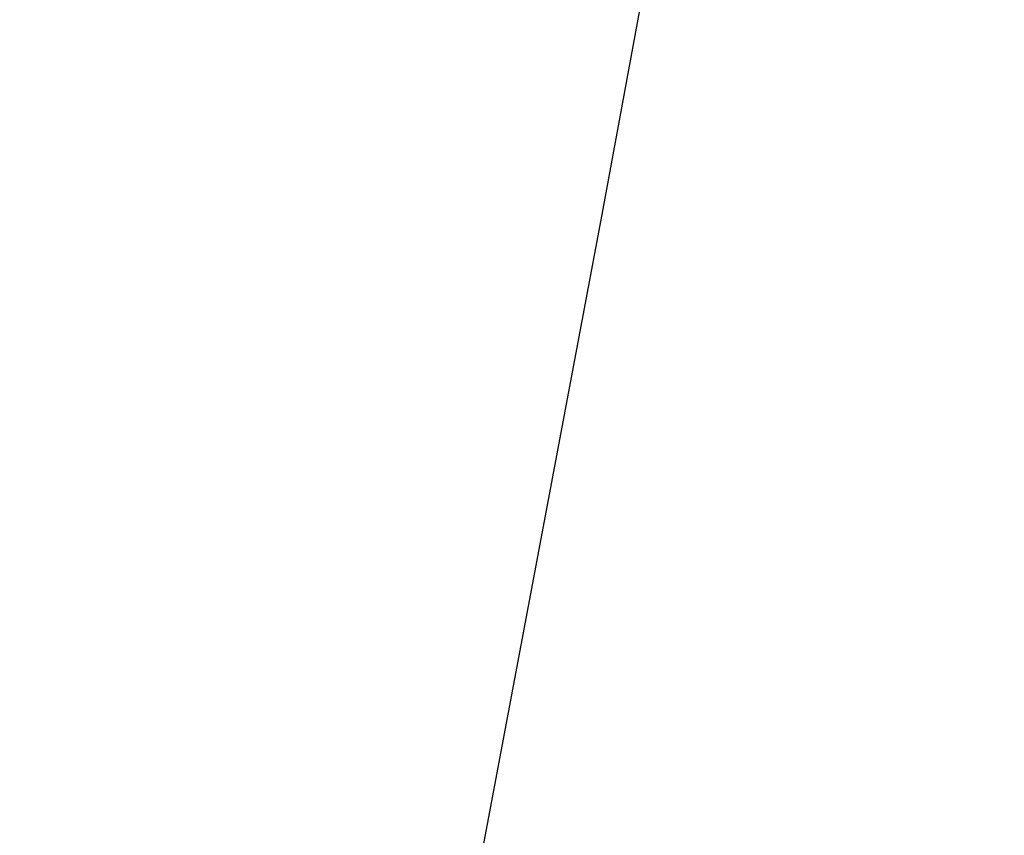
# Model space of a CAD drawing. Units: inches. Extents: x 3590 to 5167, y 65 to 1917.
# Tile 85 of 100: x 5051.4139 to 5051.6658, y 1788.8231 to 1789.0318. Entities that reach past the tile are written whole.
import ezdxf

# ---------------------------------------------------------------- set-up
doc = ezdxf.new("R2010")
doc.units = ezdxf.units.IN
doc.layers.add('A-FLOR-PATT', color=8, linetype='Continuous', lineweight=13)
doc.layers.add('L-PLNT', color=94, linetype='Continuous', lineweight=18)
doc.layers.add('DIENHOA', color=3, linetype='Continuous')

# ---------------------------------------------------------------- blocks, each defined once
blk = doc.blocks.new('Cay03_mb')
at = {"layer": 'DIENHOA'}
blk.add_lwpolyline([(87.915, 628.525), (75.456, 544.179), (61.266, 461.155), (46.129, 379.14), (30.826, 297.822), (16.139, 216.889), (2.853, 136.026), (-8.252, 54.923), (-16.392, -26.735)], dxfattribs=at)

msp = doc.modelspace()

# ---------------------------------------------------------------- hatches: boundary and pattern name
at = {"layer": 'A-FLOR-PATT', "transparency": 33554687}
h = msp.add_hatch(dxfattribs=at)
h.set_pattern_fill('AR-HBONE', color=256, scale=0.2)
h.set_pattern_definition([(45, (-588.972, 0), (0, 28.73682), [60.96, -20.32]), (135, (-574.604, 14.368), (3e-15, 28.73682), [60.96, -20.32])])
h.paths.add_polyline_path([(5071.27403, 1796.99898), (4933.27403, 1796.99898), (4933.27403, 1753.99898), (4962.77403, 1753.99898, -0.414214), (4928.77403, 1719.99898), (4933.27403, 1718.99898), (4933.27403, 1334.99898), (5071.27403, 1334.99898)])
h.paths.add_polyline_path([(4951.78002, 1521.0767), (4951.7151, 1521.0404), (4951.56345, 1520.89532)], flags=16)
h.paths.add_polyline_path([(4952.267, 1521.37645), (4952.1977, 1521.37111), (4952.19823, 1521.35558)], flags=0)
h.paths.add_polyline_path([(4967.05076, 1529.72832), (4965.23122, 1528.69444), (4963.41109, 1527.71401), (4961.75649, 1526.85081), (4963.58887, 1527.44938), (4964.03555, 1527.47802), (4962.9755, 1527.24902), (4961.76022, 1526.85203), (4959.79219, 1525.83406), (4958.00498, 1524.89483), (4956.24031, 1523.92961), (4954.50395, 1522.91854), (4954.1294, 1522.68163), (4953.36051, 1521.99688), (4953.36558, 1521.99754), (4953.605, 1522.06367), (4955.10605, 1522.76083), (4956.92108, 1523.43405), (4958.67784, 1523.91513), (4960.35834, 1524.20036), (4961.94456, 1524.28606), (4964.17144, 1524.10849), (4965.95752, 1523.30903), (4963.86273, 1522.97565), (4965.18742, 1522.49898), (4963.36614, 1522.49715), (4961.54526, 1522.48682), (4959.76359, 1522.46077), (4958.30414, 1522.4188), (4957.97356, 1522.38829), (4956.30692, 1522.2324), (4954.71821, 1522.07143), (4953.25077, 1521.89915), (4953.52509, 1521.62277), (4954.33087, 1521.37883), (4956.24263, 1521.22987), (4958.03913, 1520.92952), (4959.68424, 1520.48339), (4961.16007, 1519.89569), (4963.10699, 1518.80022), (4964.39286, 1517.32518), (4962.97306, 1517.72596), (4964.55841, 1516.66059), (4965.40664, 1515.70779), (4963.50733, 1516.32179), (4961.67995, 1517.0051), (4959.93478, 1517.74489), (4958.2821, 1518.52833), (4956.73216, 1519.34257), (4955.29527, 1520.17478), (4954.67155, 1520.57237), (4954.51279, 1520.6271), (4955.65848, 1519.31837), (4956.70263, 1517.98232), (4957.64403, 1516.64663), (4958.48545, 1515.33439), (4959.54998, 1513.52398), (4960.43768, 1511.76936), (4958.84107, 1513.6196), (4957.45175, 1515.3249), (4955.8186, 1517.45855), (4956.66537, 1515.44764), (4957.11109, 1513.92292), (4957.44681, 1511.71434), (4957.07641, 1509.79288), (4956.53757, 1511.1103), (4955.99231, 1512.56892), (4955.44448, 1514.12509), (4954.89794, 1515.73518), (4954.35653, 1517.35553), (4953.82412, 1518.94251), (4953.30455, 1520.45247), (4953.06452, 1521.11563), (4952.97143, 1521.14607), (4952.94932, 1521.08646), (4952.72981, 1520.19905), (4953.3698, 1518.02364), (4953.75708, 1516.37279), (4954.05124, 1514.76538), (4954.26449, 1513.22121), (4954.47124, 1511.13121), (4954.4971, 1510.40174), (4954.40903, 1511.76006), (4954.26449, 1513.22121), (4954.05124, 1514.76538), (4953.75708, 1516.37279), (4953.3698, 1518.02364), (4952.87718, 1519.69813), (4952.7161, 1520.1412), (4952.53301, 1519.05871), (4952.37428, 1517.78881), (4952.21925, 1516.31167), (4952.04598, 1514.59986), (4951.83253, 1512.62598), (4951.55697, 1510.36259), (4951.20331, 1512.16818), (4950.85168, 1514.33931), (4950.98529, 1516.37594), (4951.6596, 1518.28625), (4952.59261, 1520.48085), (4952.35664, 1521.1299), (4951.85502, 1520.32753), (4950.83901, 1518.90828), (4949.77675, 1517.58658), (4948.91554, 1516.61731), (4948.11099, 1515.2561), (4947.0891, 1513.55389), (4945.88937, 1511.61495), (4946.32587, 1513.40232), (4946.5624, 1514.24913), (4945.52771, 1513.32668), (4944.58105, 1512.53126), (4946.01774, 1514.50825), (4947.2044, 1516.04763), (4947.89331, 1517.31331), (4949.30686, 1518.76446), (4950.41417, 1519.76716), (4950.45131, 1519.80628), (4952.267, 1521.37645), (4951.64457, 1521.49317), (4950.40371, 1521.17954), (4948.04447, 1520.35868), (4946.11863, 1519.45198), (4944.57182, 1518.47484), (4943.34962, 1517.44265), (4941.99695, 1515.91971), (4941.66146, 1515.27475), (4942.81332, 1516.98973), (4944.57182, 1518.47484), (4946.11863, 1519.45198), (4948.04447, 1520.35868), (4950.40371, 1521.17954), (4951.64457, 1521.49317), (4949.64678, 1521.86781), (4948.59979, 1521.75633), (4947.12629, 1521.5699), (4945.42015, 1521.34763), (4943.44969, 1521.10462), (4941.18319, 1520.85596), (4942.86028, 1521.61265), (4943.87308, 1522.03014), (4942.95216, 1521.9093), (4941.40968, 1521.48512), (4939.54287, 1520.67019), (4938.96775, 1520.2255), (4940.73284, 1521.29899), (4942.95216, 1521.9093), (4943.70184, 1522.00767), (4945.89419, 1522.69998), (4947.56488, 1522.71399), (4948.92086, 1522.56573), (4951.13144, 1522.18271), (4950.97062, 1522.2969), (4948.12924, 1523.00563), (4946.03496, 1523.70671), (4944.23235, 1524.52143), (4942.70692, 1525.46111), (4941.44419, 1526.53707), (4940.42968, 1527.76062), (4939.6489, 1529.14306), (4941.42091, 1528.12232), (4943.14742, 1527.13248), (4944.84093, 1526.17457), (4946.51394, 1525.24959), (4948.17893, 1524.35855), (4948.36457, 1524.26336), (4946.47531, 1526.04459), (4945.18083, 1527.54042), (4944.19039, 1529.03339), (4943.49559, 1530.53985), (4943.27808, 1531.3597), (4942.49849, 1531.91903), (4943.11353, 1531.76249), (4942.95927, 1533.6586), (4944.13953, 1531.9886), (4944.61171, 1531.32339), (4946.20163, 1530.46341), (4947.48567, 1529.50925), (4948.79027, 1528.22649), (4950.36754, 1526.23746), (4949.48547, 1528.15549), (4948.85128, 1530.12254), (4948.49054, 1532.04127), (4948.38105, 1533.91822), (4948.50062, 1535.7599), (4948.82704, 1537.57284), (4949.41803, 1535.56526), (4949.95684, 1533.56932), (4950.46414, 1531.5861), (4950.96058, 1529.6167), (4951.3911, 1527.95448), (4951.72352, 1530.68689), (4952.20106, 1532.57994), (4952.88914, 1534.32964), (4953.77035, 1535.95123), (4954.82726, 1537.45995), (4954.52145, 1535.38966), (4954.27314, 1533.93684), (4955.57999, 1535.6627), (4956.74758, 1536.73859), (4956.15852, 1534.78029), (4955.58917, 1532.87334), (4955.04336, 1531.00581), (4954.52493, 1529.16576), (4954.03771, 1527.34127), (4953.63833, 1525.73298), (4953.61143, 1525.58564), (4953.39805, 1524.16565), (4953.38219, 1524.00887), (4954.06955, 1525.47563), (4954.91212, 1527.02173), (4956.13627, 1528.89351), (4957.84668, 1530.57701), (4959.37601, 1531.54014), (4958.25596, 1530.10398), (4957.14284, 1528.66291), (4956.06626, 1527.24305), (4955.05579, 1525.87054), (4954.14104, 1524.57149), (4953.35159, 1523.37204), (4953.31079, 1523.30299), (4953.27253, 1522.92478), (4953.26102, 1522.38213), (4954.1031, 1523.37273), (4954.63005, 1524.28376), (4955.96149, 1526.35767), (4957.23002, 1528.12969), (4958.42057, 1529.60864), (4960.03671, 1531.36792), (4961.3736, 1532.3752), (4962.1015, 1532.77), (4961.06994, 1531.06113), (4959.98733, 1529.43811), (4958.86851, 1527.90803), (4958.15046, 1527.00742), (4959.80291, 1528.00314), (4961.58854, 1528.79257), (4963.39087, 1529.32783), (4965.21118, 1529.63205)], flags=16)
h.paths.add_polyline_path([(4962.94387, 1523.18187), (4961.10714, 1523.42192), (4960.39205, 1523.36158), (4962.34964, 1523.33061)], flags=0)
h.paths.add_polyline_path([(5049.54129, 1584.55089), (5049.47636, 1584.51458), (5049.32471, 1584.3695)], flags=16)
h.paths.add_polyline_path([(5050.02827, 1584.85063), (5049.95897, 1584.84529), (5049.95949, 1584.82976)], flags=0)
h.paths.add_polyline_path([(5042.33308, 1581.94902), (5043.8799, 1582.92616), (5045.80573, 1583.83286), (5048.16498, 1584.65372), (5049.40583, 1584.96736), (5047.40804, 1585.34199), (5046.36106, 1585.23052), (5044.88755, 1585.04408), (5043.18142, 1584.82181), (5041.21095, 1584.5788), (5038.94446, 1584.33014), (5040.62155, 1585.08683), (5041.63434, 1585.50432), (5040.71343, 1585.38348), (5039.17095, 1584.9593), (5037.30414, 1584.14438), (5036.72901, 1583.69969), (5038.4941, 1584.77317), (5040.71343, 1585.38348), (5041.4631, 1585.48185), (5043.65545, 1586.17416), (5045.32615, 1586.18818), (5046.68212, 1586.03992), (5048.8927, 1585.6569), (5048.73188, 1585.77108), (5045.89051, 1586.47981), (5043.79622, 1587.18089), (5041.99361, 1587.99561), (5040.46818, 1588.9353), (5039.20546, 1590.01125), (5038.19095, 1591.2348), (5037.41016, 1592.61725), (5039.18217, 1591.5965), (5040.90868, 1590.60667), (5042.6022, 1589.64876), (5044.2752, 1588.72378), (5045.94019, 1587.83274), (5046.12584, 1587.73754), (5044.23658, 1589.51878), (5042.9421, 1591.01461), (5041.95166, 1592.50757), (5041.25685, 1594.01403), (5041.03935, 1594.83388), (5040.25976, 1595.39321), (5040.8748, 1595.23667), (5040.72054, 1597.13279), (5041.9008, 1595.46278), (5042.37297, 1594.79758), (5043.96289, 1593.93759), (5045.24694, 1592.98344), (5046.55153, 1591.70068), (5048.12881, 1589.71164), (5047.24673, 1591.62967), (5046.61254, 1593.59672), (5046.2518, 1595.51546), (5046.14232, 1597.3924), (5046.26189, 1599.23408), (5046.5883, 1601.04703), (5047.17929, 1599.03944), (5047.71811, 1597.0435), (5048.22541, 1595.06028), (5048.72184, 1593.09089), (5049.15237, 1591.42866), (5049.48478, 1594.16107), (5049.96233, 1596.05412), (5050.65041, 1597.80382), (5051.53161, 1599.42541), (5052.58852, 1600.93414), (5052.28271, 1598.86384), (5052.03441, 1597.41102), (5053.34126, 1599.13689), (5054.50884, 1600.21277), (5053.91979, 1598.25447), (5053.35044, 1596.34752), (5052.80463, 1594.47999), (5052.2862, 1592.63995), (5051.79898, 1590.81546), (5051.39959, 1589.20716), (5051.3727, 1589.05983), (5051.15931, 1587.63984), (5051.14346, 1587.48305), (5051.83082, 1588.94982), (5052.67339, 1590.49592), (5053.89754, 1592.3677), (5055.60794, 1594.05119), (5057.13728, 1595.01432), (5056.01722, 1593.57817), (5054.90411, 1592.1371), (5053.82752, 1590.71724), (5052.81705, 1589.34472), (5051.9023, 1588.04567), (5051.11286, 1586.84622), (5051.07205, 1586.77718), (5051.03379, 1586.39896), (5051.02228, 1585.85631), (5051.86437, 1586.84692), (5052.39131, 1587.75794), (5053.72275, 1589.83185), (5054.99128, 1591.60387), (5056.18183, 1593.08282), (5057.79798, 1594.84211), (5059.13486, 1595.84938), (5059.86276, 1596.24419), (5058.83121, 1594.53531), (5057.7486, 1592.9123), (5056.62978, 1591.38221), (5055.91173, 1590.4816), (5057.56418, 1591.47732), (5059.34981, 1592.26675), (5061.15214, 1592.80202), (5062.97245, 1593.10624), (5064.81203, 1593.20251), (5062.99248, 1592.16863), (5061.17235, 1591.18819), (5059.51775, 1590.325), (5061.35014, 1590.92356), (5061.79682, 1590.95221), (5060.73676, 1590.7232), (5059.52148, 1590.32622), (5057.55345, 1589.30825), (5055.76625, 1588.36901), (5054.00157, 1587.40379), (5052.26521, 1586.39273), (5051.89067, 1586.15581), (5051.12177, 1585.47106), (5051.12684, 1585.47172), (5051.36627, 1585.53786), (5052.86732, 1586.23502), (5054.68234, 1586.90824), (5056.4391, 1587.38931), (5058.1196, 1587.67454), (5059.70582, 1587.76024), (5061.93271, 1587.58268), (5063.71878, 1586.78321), (5061.62399, 1586.44983), (5062.94869, 1585.97317), (5061.12741, 1585.97133), (5059.30653, 1585.961), (5057.52486, 1585.93496), (5056.06541, 1585.89299), (5055.73482, 1585.86247), (5054.06819, 1585.70658), (5052.47947, 1585.54561), (5051.01204, 1585.37333), (5051.28635, 1585.09695), (5052.09214, 1584.85301), (5054.00389, 1584.70406), (5055.8004, 1584.4037), (5057.44551, 1583.95757), (5058.92133, 1583.36987), (5060.86825, 1582.27441), (5062.15413, 1580.79937), (5060.73433, 1581.20015), (5062.31967, 1580.13477), (5063.1679, 1579.18198), (5061.2686, 1579.79597), (5059.44122, 1580.47928), (5057.69605, 1581.21908), (5056.04336, 1582.00251), (5054.49343, 1582.81675), (5053.05653, 1583.64897), (5052.43281, 1584.04656), (5052.27405, 1584.10128), (5053.41974, 1582.79255), (5054.4639, 1581.4565), (5055.40529, 1580.12081), (5056.24672, 1578.80858), (5057.31125, 1576.99816), (5058.19895, 1575.24354), (5056.60234, 1577.09378), (5055.21301, 1578.79908), (5053.57987, 1580.93274), (5054.42664, 1578.92183), (5054.87235, 1577.3971), (5055.20808, 1575.18852), (5054.83767, 1573.26706), (5054.29883, 1574.58448), (5053.75357, 1576.0431), (5053.20575, 1577.59927), (5052.6592, 1579.20936), (5052.1178, 1580.82971), (5051.58538, 1582.41669), (5051.06582, 1583.92666), (5050.82578, 1584.58981), (5050.7327, 1584.62025), (5050.71058, 1584.56064), (5050.49108, 1583.67323), (5051.13107, 1581.49782), (5051.51835, 1579.84698), (5051.8125, 1578.23957), (5052.02575, 1576.69539), (5052.23251, 1574.6054), (5052.25836, 1573.87593), (5052.1703, 1575.23424), (5052.02575, 1576.69539), (5051.8125, 1578.23957), (5051.51835, 1579.84698), (5051.13107, 1581.49782), (5050.63844, 1583.17231), (5050.47736, 1583.61538), (5050.29428, 1582.53289), (5050.13554, 1581.26299), (5049.98051, 1579.78585), (5049.80724, 1578.07405), (5049.59379, 1576.10016), (5049.31823, 1573.83678), (5048.96458, 1575.64237), (5048.61294, 1577.8135), (5048.74656, 1579.85012), (5049.42086, 1581.76043), (5050.35388, 1583.95503), (5050.1179, 1584.60408), (5049.61629, 1583.80172), (5048.60027, 1582.38246), (5047.53801, 1581.06076), (5046.67681, 1580.09149), (5045.87225, 1578.73029), (5044.85036, 1577.02808), (5043.65063, 1575.08913), (5044.08713, 1576.8765), (5044.32366, 1577.72331), (5043.28898, 1576.80086), (5042.34232, 1576.00545), (5043.779, 1577.98243), (5044.96566, 1579.52182), (5045.65457, 1580.78749), (5047.06813, 1582.23865), (5048.17543, 1583.24134), (5048.21258, 1583.28047), (5050.02827, 1584.85063), (5049.40583, 1584.96736), (5048.16498, 1584.65372), (5045.80573, 1583.83286), (5043.8799, 1582.92616), (5042.33308, 1581.94902), (5041.11088, 1580.91684), (5039.75821, 1579.39389), (5039.42272, 1578.74894), (5040.57458, 1580.46391)], flags=16)
h.paths.add_polyline_path([(4954.79872, 1533.12029), (4954.26249, 1532.07935), (4953.83112, 1530.93464), (4953.50472, 1529.63602), (4953.28338, 1528.13331), (4953.16721, 1526.37637), (4953.15631, 1524.31504), (4953.27669, 1521.23629), (4952.80168, 1521.84177), (4951.55695, 1521.99789), (4950.97575, 1521.9613), (4952.66059, 1521.94097), (4952.80168, 1521.84177), (4953.15249, 1523.59258), (4953.16721, 1526.37637), (4953.28338, 1528.13331), (4953.60929, 1530.34598), (4954.45558, 1532.59174)], flags=0)
h.paths.add_polyline_path([(5050.56294, 1585.31596), (5049.31822, 1585.47208), (5048.73702, 1585.43548), (5050.42186, 1585.41516), (5050.56294, 1585.31596), (5050.91375, 1587.06676), (5050.92848, 1589.85056), (5051.04465, 1591.6075), (5051.37055, 1593.82017), (5052.21684, 1596.06593), (5052.55999, 1596.59447), (5052.02375, 1595.55353), (5051.59238, 1594.40883), (5051.26598, 1593.1102), (5051.04465, 1591.6075), (5050.92848, 1589.85056), (5050.91757, 1587.78922), (5051.03795, 1584.71048)], flags=0)
h.paths.add_polyline_path([(5058.15332, 1586.83576), (5060.11091, 1586.80479), (5060.70514, 1586.65605), (5058.8684, 1586.8961)], flags=0)
h.paths.add_polyline_path([(5049.54129, 1430.93611), (5049.47636, 1430.8998), (5049.32471, 1430.75472)], flags=16)
h.paths.add_polyline_path([(5050.02827, 1431.23585), (5049.95897, 1431.23051), (5049.95949, 1431.21498)], flags=0)
h.paths.add_polyline_path([(5046.5883, 1447.43225), (5047.17929, 1445.42467), (5047.71811, 1443.42872), (5048.22541, 1441.4455), (5048.72184, 1439.47611), (5049.15237, 1437.81388), (5049.48478, 1440.5463), (5049.96233, 1442.43934), (5050.65041, 1444.18904), (5051.53161, 1445.81063), (5052.58852, 1447.31936), (5052.28271, 1445.24906), (5052.03441, 1443.79624), (5053.34126, 1445.52211), (5054.50884, 1446.59799), (5053.91979, 1444.63969), (5053.35044, 1442.73274), (5052.80463, 1440.86521), (5052.2862, 1439.02517), (5051.79898, 1437.20068), (5051.39959, 1435.59238), (5051.3727, 1435.44505), (5051.15931, 1434.02506), (5051.14346, 1433.86828), (5051.83082, 1435.33504), (5052.67339, 1436.88114), (5053.89754, 1438.75292), (5055.60794, 1440.43641), (5057.13728, 1441.39954), (5056.01722, 1439.96339), (5054.90411, 1438.52232), (5053.82752, 1437.10246), (5052.81705, 1435.72994), (5051.9023, 1434.4309), (5051.11286, 1433.23145), (5051.07205, 1433.1624), (5051.03379, 1432.78418), (5051.02228, 1432.24153), (5051.86437, 1433.23214), (5052.39131, 1434.14316), (5053.72275, 1436.21707), (5054.99128, 1437.98909), (5056.18183, 1439.46805), (5057.79798, 1441.22733), (5059.13486, 1442.23461), (5059.86276, 1442.62941), (5058.83121, 1440.92053), (5057.7486, 1439.29752), (5056.62978, 1437.76743), (5055.91173, 1436.86682), (5057.56418, 1437.86255), (5059.34981, 1438.65197), (5061.15214, 1439.18724), (5062.97245, 1439.49146), (5064.81203, 1439.58773), (5062.99248, 1438.55385), (5061.17235, 1437.57342), (5059.51775, 1436.71022), (5061.35014, 1437.30879), (5061.79682, 1437.33743), (5060.73676, 1437.10842), (5059.52148, 1436.71144), (5057.55345, 1435.69347), (5055.76625, 1434.75423), (5054.00157, 1433.78901), (5052.26521, 1432.77795), (5051.89067, 1432.54103), (5051.12177, 1431.85628), (5051.12684, 1431.85694), (5051.36627, 1431.92308), (5052.86732, 1432.62024), (5054.68234, 1433.29346), (5056.4391, 1433.77453), (5058.1196, 1434.05976), (5059.70582, 1434.14546), (5061.93271, 1433.9679), (5063.71878, 1433.16843), (5061.62399, 1432.83505), (5062.94869, 1432.35839), (5061.12741, 1432.35655), (5059.30653, 1432.34623), (5057.52486, 1432.32018), (5056.06541, 1432.27821), (5055.73482, 1432.24769), (5054.06819, 1432.09181), (5052.47947, 1431.93083), (5051.01204, 1431.75856), (5051.28635, 1431.48218), (5052.09214, 1431.23823), (5054.00389, 1431.08928), (5055.8004, 1430.78892), (5057.44551, 1430.34279), (5058.92133, 1429.75509), (5060.86825, 1428.65963), (5062.15413, 1427.18459), (5060.73433, 1427.58537), (5062.31967, 1426.52), (5063.1679, 1425.5672), (5061.2686, 1426.18119), (5059.44122, 1426.86451), (5057.69605, 1427.6043), (5056.04336, 1428.38773), (5054.49343, 1429.20197), (5053.05653, 1430.03419), (5052.43281, 1430.43178), (5052.27405, 1430.48651), (5053.41974, 1429.17777), (5054.4639, 1427.84172), (5055.40529, 1426.50603), (5056.24672, 1425.1938), (5057.31125, 1423.38338), (5058.19895, 1421.62877), (5056.60234, 1423.479), (5055.21301, 1425.1843), (5053.57987, 1427.31796), (5054.42664, 1425.30705), (5054.87235, 1423.78233), (5055.20808, 1421.57374), (5054.83767, 1419.65228), (5054.29883, 1420.9697), (5053.75357, 1422.42832), (5053.20575, 1423.9845), (5052.6592, 1425.59458), (5052.1178, 1427.21493), (5051.58538, 1428.80191), (5051.06582, 1430.31188), (5050.82578, 1430.97503), (5050.7327, 1431.00547), (5050.71058, 1430.94586), (5050.49108, 1430.05845), (5051.13107, 1427.88305), (5051.51835, 1426.2322), (5051.8125, 1424.62479), (5052.02575, 1423.08061), (5052.23251, 1420.99062), (5052.25836, 1420.26115), (5052.1703, 1421.61947), (5052.02575, 1423.08061), (5051.8125, 1424.62479), (5051.51835, 1426.2322), (5051.13107, 1427.88305), (5050.63844, 1429.55753), (5050.47736, 1430.0006), (5050.29428, 1428.91811), (5050.13554, 1427.64821), (5049.98051, 1426.17107), (5049.80724, 1424.45927), (5049.59379, 1422.48539), (5049.31823, 1420.222), (5048.96458, 1422.02759), (5048.61294, 1424.19872), (5048.74656, 1426.23534), (5049.42086, 1428.14565), (5050.35388, 1430.34025), (5050.1179, 1430.98931), (5049.61629, 1430.18694), (5048.60027, 1428.76768), (5047.53801, 1427.44598), (5046.67681, 1426.47671), (5045.87225, 1425.11551), (5044.85036, 1423.4133), (5043.65063, 1421.47435), (5044.08713, 1423.26172), (5044.32366, 1424.10854), (5043.28898, 1423.18608), (5042.34232, 1422.39067), (5043.779, 1424.36765), (5044.96566, 1425.90704), (5045.65457, 1427.17272), (5047.06813, 1428.62387), (5048.17543, 1429.62657), (5048.21258, 1429.66569), (5050.02827, 1431.23585), (5049.40583, 1431.35258), (5048.16498, 1431.03894), (5045.80573, 1430.21809), (5043.8799, 1429.31139), (5042.33308, 1428.33424), (5041.11088, 1427.30206), (5039.75821, 1425.77911), (5039.42272, 1425.13416), (5040.57458, 1426.84914), (5042.33308, 1428.33424), (5043.8799, 1429.31139), (5045.80573, 1430.21809), (5048.16498, 1431.03894), (5049.40583, 1431.35258), (5047.40804, 1431.72722), (5046.36106, 1431.61574), (5044.88755, 1431.42931), (5043.18142, 1431.20704), (5041.21095, 1430.96402), (5038.94446, 1430.71536), (5040.62155, 1431.47205), (5041.63434, 1431.88954), (5040.71343, 1431.76871), (5039.17095, 1431.34453), (5037.30414, 1430.5296), (5036.72901, 1430.08491), (5038.4941, 1431.1584), (5040.71343, 1431.76871), (5041.4631, 1431.86707), (5043.65545, 1432.55939), (5045.32615, 1432.5734), (5046.68212, 1432.42514), (5048.8927, 1432.04212), (5048.73188, 1432.1563), (5045.89051, 1432.86503), (5043.79622, 1433.56611), (5041.99361, 1434.38083), (5040.46818, 1435.32052), (5039.20546, 1436.39648), (5038.19095, 1437.62002), (5037.41016, 1439.00247), (5039.18217, 1437.98172), (5040.90868, 1436.99189), (5042.6022, 1436.03398), (5044.2752, 1435.109), (5045.94019, 1434.21796), (5046.12584, 1434.12276), (5044.23658, 1435.904), (5042.9421, 1437.39983), (5041.95166, 1438.8928), (5041.25685, 1440.39925), (5041.03935, 1441.2191), (5040.25976, 1441.77844), (5040.8748, 1441.62189), (5040.72054, 1443.51801), (5041.9008, 1441.848), (5042.37297, 1441.1828), (5043.96289, 1440.32282), (5045.24694, 1439.36866), (5046.55153, 1438.0859), (5048.12881, 1436.09686), (5047.24673, 1438.01489), (5046.61254, 1439.98195), (5046.2518, 1441.90068), (5046.14232, 1443.77762), (5046.26189, 1445.6193)], flags=16)
h.paths.add_polyline_path([(5052.38176, 1444.25496), (5051.62263, 1442.77987), (5052.02375, 1441.93875), (5052.55999, 1442.9797)], flags=0)
h.paths.add_polyline_path([(5050.56294, 1431.70118), (5049.31822, 1431.8573), (5048.73702, 1431.82071), (5050.42186, 1431.80038)], flags=0)
h.paths.add_polyline_path([(5058.15332, 1433.22098), (5060.11091, 1433.19001), (5060.70514, 1433.04127), (5058.8684, 1433.28132)], flags=0)
h.paths.add_polyline_path([(5049.54129, 1352.28535), (5049.47636, 1352.24904), (5049.32471, 1352.10396)], flags=16)
h.paths.add_polyline_path([(5050.02827, 1352.58509), (5049.95897, 1352.57975), (5049.95949, 1352.56422)], flags=0)
h.paths.add_polyline_path([(5046.5883, 1368.78149), (5047.17929, 1366.7739), (5047.71811, 1364.77796), (5048.22541, 1362.79474), (5048.72184, 1360.82534), (5049.15237, 1359.16312), (5049.48478, 1361.89553), (5049.96233, 1363.78858), (5050.65041, 1365.53828), (5051.53161, 1367.15987), (5052.58852, 1368.6686), (5052.28271, 1366.5983), (5052.03441, 1365.14548), (5053.34126, 1366.87135), (5054.50884, 1367.94723), (5053.91979, 1365.98893), (5053.35044, 1364.08198), (5052.80463, 1362.21445), (5052.2862, 1360.37441), (5051.79898, 1358.54992), (5051.39959, 1356.94162), (5051.3727, 1356.79428), (5051.15931, 1355.37429), (5051.14346, 1355.21751), (5051.83082, 1356.68428), (5052.67339, 1358.23037), (5053.89754, 1360.10216), (5055.60794, 1361.78565), (5057.13728, 1362.74878), (5056.01722, 1361.31262), (5054.90411, 1359.87155), (5053.82752, 1358.4517), (5052.81705, 1357.07918), (5051.9023, 1355.78013), (5051.11286, 1354.58068), (5051.07205, 1354.51164), (5051.03379, 1354.13342), (5051.02228, 1353.59077), (5051.86437, 1354.58137), (5052.39131, 1355.4924), (5053.72275, 1357.56631), (5054.99128, 1359.33833), (5056.18183, 1360.81728), (5057.79798, 1362.57656), (5059.13486, 1363.58384), (5059.86276, 1363.97864), (5058.83121, 1362.26977), (5057.7486, 1360.64675), (5056.62978, 1359.11667), (5055.91173, 1358.21606), (5057.56418, 1359.21178), (5059.34981, 1360.00121), (5061.15214, 1360.53648), (5062.97245, 1360.84069), (5064.81203, 1360.93697), (5062.99248, 1359.90308), (5061.17235, 1358.92265), (5059.51775, 1358.05946), (5061.35014, 1358.65802), (5061.79682, 1358.68666), (5060.73676, 1358.45766), (5059.52148, 1358.06068), (5057.55345, 1357.0427), (5055.76625, 1356.10347), (5054.00157, 1355.13825), (5052.26521, 1354.12718), (5051.89067, 1353.89027), (5051.12177, 1353.20552), (5051.12684, 1353.20618), (5051.36627, 1353.27231), (5052.86732, 1353.96947), (5054.68234, 1354.6427), (5056.4391, 1355.12377), (5058.1196, 1355.409), (5059.70582, 1355.4947), (5061.93271, 1355.31713), (5063.71878, 1354.51767), (5061.62399, 1354.18429), (5062.94869, 1353.70763), (5061.12741, 1353.70579), (5059.30653, 1353.69546), (5057.52486, 1353.66942), (5056.06541, 1353.62744), (5055.73482, 1353.59693), (5054.06819, 1353.44104), (5052.47947, 1353.28007), (5051.01204, 1353.10779), (5051.28635, 1352.83141), (5052.09214, 1352.58747), (5054.00389, 1352.43852), (5055.8004, 1352.13816), (5057.44551, 1351.69203), (5058.92133, 1351.10433), (5060.86825, 1350.00887), (5062.15413, 1348.53382), (5060.73433, 1348.9346), (5062.31967, 1347.86923), (5063.1679, 1346.91643), (5061.2686, 1347.53043), (5059.44122, 1348.21374), (5057.69605, 1348.95353), (5056.04336, 1349.73697), (5054.49343, 1350.55121), (5053.05653, 1351.38342), (5052.43281, 1351.78101), (5052.27405, 1351.83574), (5053.41974, 1350.52701), (5054.4639, 1349.19096), (5055.40529, 1347.85527), (5056.24672, 1346.54303), (5057.31125, 1344.73262), (5058.19895, 1342.978), (5056.60234, 1344.82824), (5055.21301, 1346.53354), (5053.57987, 1348.6672), (5054.42664, 1346.65629), (5054.87235, 1345.13156), (5055.20808, 1342.92298), (5054.83767, 1341.00152), (5054.29883, 1342.31894), (5053.75357, 1343.77756), (5053.20575, 1345.33373), (5052.6592, 1346.94382), (5052.1178, 1348.56417), (5051.58538, 1350.15115), (5051.06582, 1351.66111), (5050.82578, 1352.32427), (5050.7327, 1352.35471), (5050.71058, 1352.2951), (5050.49108, 1351.40769), (5051.13107, 1349.23228), (5051.51835, 1347.58144), (5051.8125, 1345.97403), (5052.02575, 1344.42985), (5052.23251, 1342.33986), (5052.25836, 1341.61039), (5052.1703, 1342.9687), (5052.02575, 1344.42985), (5051.8125, 1345.97403), (5051.51835, 1347.58144), (5051.13107, 1349.23228), (5050.63844, 1350.90677), (5050.47736, 1351.34984), (5050.29428, 1350.26735), (5050.13554, 1348.99745), (5049.98051, 1347.52031), (5049.80724, 1345.80851), (5049.59379, 1343.83462), (5049.31823, 1341.57124), (5048.96458, 1343.37683), (5048.61294, 1345.54796), (5048.74656, 1347.58458), (5049.42086, 1349.49489), (5050.35388, 1351.68949), (5050.1179, 1352.33854), (5049.61629, 1351.53617), (5048.60027, 1350.11692), (5047.53801, 1348.79522), (5046.67681, 1347.82595), (5045.87225, 1346.46475), (5044.85036, 1344.76253), (5043.65063, 1342.82359), (5044.08713, 1344.61096), (5044.32366, 1345.45777), (5043.28898, 1344.53532), (5042.34232, 1343.7399), (5043.779, 1345.71689), (5044.96566, 1347.25627), (5045.65457, 1348.52195), (5047.06813, 1349.9731), (5048.17543, 1350.9758), (5048.21258, 1351.01493), (5050.02827, 1352.58509), (5049.40583, 1352.70181), (5048.16498, 1352.38818), (5045.80573, 1351.56732), (5043.8799, 1350.66062), (5042.33308, 1349.68348), (5041.11088, 1348.65129), (5039.75821, 1347.12835), (5039.42272, 1346.4834), (5040.57458, 1348.19837), (5042.33308, 1349.68348), (5043.8799, 1350.66062), (5045.80573, 1351.56732), (5048.16498, 1352.38818), (5049.40583, 1352.70181), (5047.40804, 1353.07645), (5046.36106, 1352.96498), (5044.88755, 1352.77854), (5043.18142, 1352.55627), (5041.21095, 1352.31326), (5038.94446, 1352.0646), (5040.62155, 1352.82129), (5041.63434, 1353.23878), (5040.71343, 1353.11794), (5039.17095, 1352.69376), (5037.30414, 1351.87884), (5036.72901, 1351.43415), (5038.4941, 1352.50763), (5040.71343, 1353.11794), (5041.4631, 1353.21631), (5043.65545, 1353.90862), (5045.32615, 1353.92263), (5046.68212, 1353.77438), (5048.8927, 1353.39136), (5048.73188, 1353.50554), (5045.89051, 1354.21427), (5043.79622, 1354.91535), (5041.99361, 1355.73007), (5040.46818, 1356.66975), (5039.20546, 1357.74571), (5038.19095, 1358.96926), (5037.41016, 1360.35171), (5039.18217, 1359.33096), (5040.90868, 1358.34112), (5042.6022, 1357.38321), (5044.2752, 1356.45824), (5045.94019, 1355.5672), (5046.12584, 1355.472), (5044.23658, 1357.25323), (5042.9421, 1358.74906), (5041.95166, 1360.24203), (5041.25685, 1361.74849), (5041.03935, 1362.56834), (5040.25976, 1363.12767), (5040.8748, 1362.97113), (5040.72054, 1364.86725), (5041.9008, 1363.19724), (5042.37297, 1362.53203), (5043.96289, 1361.67205), (5045.24694, 1360.7179), (5046.55153, 1359.43513), (5048.12881, 1357.4461), (5047.24673, 1359.36413), (5046.61254, 1361.33118), (5046.2518, 1363.24992), (5046.14232, 1365.12686), (5046.26189, 1366.96854)], flags=16)
h.paths.add_polyline_path([(5052.38176, 1365.6042), (5051.62263, 1364.12911), (5052.02375, 1363.28799), (5052.55999, 1364.32893)], flags=0)
h.paths.add_polyline_path([(4951.78002, 1698.04081), (4951.7151, 1698.0045), (4951.56345, 1697.85942)], flags=16)
h.paths.add_polyline_path([(4952.267, 1698.34055), (4952.1977, 1698.33521), (4952.19823, 1698.31968)], flags=0)
h.paths.add_polyline_path([(4957.07641, 1686.75698), (4956.53757, 1688.0744), (4955.99231, 1689.53302), (4955.44448, 1691.08919), (4954.89794, 1692.69928), (4954.35653, 1694.31963), (4953.82412, 1695.90661), (4953.30455, 1697.41658), (4953.06452, 1698.07973), (4952.97143, 1698.11017), (4952.94932, 1698.05056), (4952.72981, 1697.16315), (4953.3698, 1694.98774), (4953.75708, 1693.3369), (4954.05124, 1691.72949), (4954.26449, 1690.18531), (4954.47124, 1688.09532), (4954.4971, 1687.36585), (4954.40903, 1688.72416), (4954.26449, 1690.18531), (4954.05124, 1691.72949), (4953.75708, 1693.3369), (4953.3698, 1694.98774), (4952.87718, 1696.66223), (4952.7161, 1697.1053), (4952.53301, 1696.02281), (4952.37428, 1694.75291), (4952.21925, 1693.27577), (4952.04598, 1691.56397), (4951.83253, 1689.59008), (4951.55697, 1687.3267), (4951.20331, 1689.13229), (4950.85168, 1691.30342), (4950.98529, 1693.34004), (4951.6596, 1695.25035), (4952.59261, 1697.44495), (4952.35664, 1698.09401), (4951.85502, 1697.29164), (4950.83901, 1695.87238), (4949.77675, 1694.55068), (4948.91554, 1693.58141), (4948.11099, 1692.22021), (4947.0891, 1690.518), (4945.88937, 1688.57905), (4946.32587, 1690.36642), (4946.5624, 1691.21323), (4945.52771, 1690.29078), (4944.58105, 1689.49537), (4946.01774, 1691.47235), (4947.2044, 1693.01174), (4947.89331, 1694.27741), (4949.30686, 1695.72857), (4950.41417, 1696.73127), (4950.45131, 1696.77039), (4952.267, 1698.34055), (4951.64457, 1698.45728), (4950.40371, 1698.14364), (4948.04447, 1697.32278), (4946.11863, 1696.41608), (4944.57182, 1695.43894), (4943.34962, 1694.40676), (4941.99695, 1692.88381), (4941.66146, 1692.23886), (4942.81332, 1693.95383), (4944.57182, 1695.43894), (4946.11863, 1696.41608), (4948.04447, 1697.32278), (4950.40371, 1698.14364), (4951.64457, 1698.45728), (4949.64678, 1698.83191), (4948.59979, 1698.72044), (4947.12629, 1698.53401), (4945.42015, 1698.31174), (4943.44969, 1698.06872), (4941.18319, 1697.82006), (4942.86028, 1698.57675), (4943.87308, 1698.99424), (4942.95216, 1698.8734), (4941.40968, 1698.44922), (4939.54287, 1697.6343), (4938.96775, 1697.18961), (4940.73284, 1698.26309), (4942.95216, 1698.8734), (4943.70184, 1698.97177), (4945.89419, 1699.66409), (4947.56488, 1699.6781), (4948.92086, 1699.52984), (4951.13144, 1699.14682), (4950.97062, 1699.261), (4948.12924, 1699.96973), (4946.03496, 1700.67081), (4944.23235, 1701.48553), (4942.70692, 1702.42522), (4941.44419, 1703.50117), (4940.42968, 1704.72472), (4939.6489, 1706.10717), (4941.42091, 1705.08642), (4943.14742, 1704.09659), (4944.84093, 1703.13868), (4946.51394, 1702.2137), (4948.17893, 1701.32266), (4948.36457, 1701.22746), (4946.47531, 1703.0087), (4945.18083, 1704.50453), (4944.19039, 1705.9975), (4943.49559, 1707.50395), (4943.27808, 1708.3238), (4942.49849, 1708.88314), (4943.11353, 1708.72659), (4942.95927, 1710.62271), (4944.13953, 1708.9527), (4944.61171, 1708.2875), (4946.20163, 1707.42751), (4947.48567, 1706.47336), (4948.79027, 1705.1906), (4950.36754, 1703.20156), (4949.48547, 1705.11959), (4948.85128, 1707.08664), (4948.49054, 1709.00538), (4948.38105, 1710.88232), (4948.50062, 1712.724), (4948.82704, 1714.53695), (4949.41803, 1712.52937), (4949.95684, 1710.53342), (4950.46414, 1708.5502), (4950.96058, 1706.58081), (4951.3911, 1704.91858), (4951.72352, 1707.65099), (4952.20106, 1709.54404), (4952.88914, 1711.29374), (4953.77035, 1712.91533), (4954.82726, 1714.42406), (4954.52145, 1712.35376), (4954.27314, 1710.90094), (4955.57999, 1712.62681), (4956.74758, 1713.70269), (4956.15852, 1711.74439), (4955.58917, 1709.83744), (4955.04336, 1707.96991), (4954.52493, 1706.12987), (4954.03771, 1704.30538), (4953.63833, 1702.69708), (4953.61143, 1702.54975), (4953.39805, 1701.12976), (4953.38219, 1700.97297), (4954.06955, 1702.43974), (4954.91212, 1703.98584), (4956.13627, 1705.85762), (4957.84668, 1707.54111), (4959.37601, 1708.50424), (4958.25596, 1707.06809), (4957.14284, 1705.62702), (4956.06626, 1704.20716), (4955.05579, 1702.83464), (4954.14104, 1701.53559), (4953.35159, 1700.33614), (4953.31079, 1700.2671), (4953.27253, 1699.88888), (4953.26102, 1699.34623), (4954.1031, 1700.33684), (4954.63005, 1701.24786), (4955.96149, 1703.32177), (4957.23002, 1705.09379), (4958.42057, 1706.57274), (4960.03671, 1708.33203), (4961.3736, 1709.33931), (4962.1015, 1709.73411), (4961.06994, 1708.02523), (4959.98733, 1706.40222), (4958.86851, 1704.87213), (4958.15046, 1703.97152), (4959.80291, 1704.96725), (4961.58854, 1705.75667), (4963.39087, 1706.29194), (4965.21118, 1706.59616), (4967.05076, 1706.69243), (4965.23122, 1705.65855), (4963.41109, 1704.67811), (4961.75649, 1703.81492), (4963.58887, 1704.41349), (4964.03555, 1704.44213), (4962.9755, 1704.21312), (4961.76022, 1703.81614), (4959.79219, 1702.79817), (4958.00498, 1701.85893), (4956.24031, 1700.89371), (4954.50395, 1699.88265), (4954.1294, 1699.64573), (4953.36051, 1698.96098), (4953.36558, 1698.96164), (4953.605, 1699.02778), (4955.10605, 1699.72494), (4956.92108, 1700.39816), (4958.67784, 1700.87923), (4960.35834, 1701.16446), (4961.94456, 1701.25016), (4964.17144, 1701.0726), (4965.95752, 1700.27313), (4963.86273, 1699.93975), (4965.18742, 1699.46309), (4963.36614, 1699.46125), (4961.54526, 1699.45092), (4959.76359, 1699.42488), (4958.30414, 1699.38291), (4957.97356, 1699.35239), (4956.30692, 1699.1965), (4954.71821, 1699.03553), (4953.25077, 1698.86326), (4953.52509, 1698.58688), (4954.33087, 1698.34293), (4956.24263, 1698.19398), (4958.03913, 1697.89362), (4959.68424, 1697.44749), (4961.16007, 1696.85979), (4963.10699, 1695.76433), (4964.39286, 1694.28929), (4962.97306, 1694.69007), (4964.55841, 1693.6247), (4965.40664, 1692.6719), (4963.50733, 1693.28589), (4961.67995, 1693.9692), (4959.93478, 1694.709), (4958.2821, 1695.49243), (4956.73216, 1696.30667), (4955.29527, 1697.13889), (4954.67155, 1697.53648), (4954.51279, 1697.5912), (4955.65848, 1696.28247), (4956.70263, 1694.94642), (4957.64403, 1693.61073), (4958.48545, 1692.2985), (4959.54998, 1690.48808), (4960.43768, 1688.73346), (4958.84107, 1690.5837), (4957.45175, 1692.289), (4955.8186, 1694.42266), (4956.66537, 1692.41175), (4957.11109, 1690.88702), (4957.44681, 1688.67844)], flags=16)
h.paths.add_polyline_path([(5050.56294, 1353.05042), (5049.31822, 1353.20654), (5048.73702, 1353.16994), (5050.42186, 1353.14961)], flags=0)
h.paths.add_polyline_path([(4951.78002, 1351.48609), (4951.7151, 1351.44979), (4951.56345, 1351.30471)], flags=16)
h.paths.add_polyline_path([(4952.267, 1351.78584), (4952.1977, 1351.7805), (4952.19823, 1351.76497)], flags=0)
h.paths.add_polyline_path([(4954.82726, 1367.86934), (4954.52145, 1365.79905), (4954.27314, 1364.34623), (4955.57999, 1366.07209), (4956.74758, 1367.14798), (4956.15852, 1365.18968), (4955.58917, 1363.28273), (4955.04336, 1361.4152), (4954.52493, 1359.57515), (4954.03771, 1357.75066), (4953.63833, 1356.14237), (4953.61143, 1355.99503), (4953.39805, 1354.57504), (4953.38219, 1354.41826), (4954.06955, 1355.88503), (4954.91212, 1357.43112), (4956.13627, 1359.3029), (4957.84668, 1360.9864), (4959.37601, 1361.94953), (4958.25596, 1360.51337), (4957.14284, 1359.0723), (4956.06626, 1357.65245), (4955.05579, 1356.27993), (4954.14104, 1354.98088), (4953.35159, 1353.78143), (4953.31079, 1353.71238), (4953.27253, 1353.33417), (4953.26102, 1352.79152), (4954.1031, 1353.78212), (4954.63005, 1354.69315), (4955.96149, 1356.76706), (4957.23002, 1358.53908), (4958.42057, 1360.01803), (4960.03671, 1361.77731), (4961.3736, 1362.78459), (4962.1015, 1363.17939), (4961.06994, 1361.47052), (4959.98733, 1359.8475), (4958.86851, 1358.31742), (4958.15046, 1357.41681), (4959.80291, 1358.41253), (4961.58854, 1359.20196), (4963.39087, 1359.73723), (4965.21118, 1360.04144), (4967.05076, 1360.13771), (4965.23122, 1359.10383), (4963.41109, 1358.1234), (4961.75649, 1357.26021), (4963.58887, 1357.85877), (4964.03555, 1357.88741), (4962.9755, 1357.65841), (4961.76022, 1357.26143), (4959.79219, 1356.24345), (4958.00498, 1355.30422), (4956.24031, 1354.339), (4954.50395, 1353.32793), (4954.1294, 1353.09102), (4953.36051, 1352.40627), (4953.36558, 1352.40693), (4953.605, 1352.47306), (4955.10605, 1353.17022), (4956.92108, 1353.84345), (4958.67784, 1354.32452), (4960.35834, 1354.60975), (4961.94456, 1354.69545), (4964.17144, 1354.51788), (4965.95752, 1353.71842), (4963.86273, 1353.38504), (4965.18742, 1352.90838), (4963.36614, 1352.90654), (4961.54526, 1352.89621), (4959.76359, 1352.87016), (4958.30414, 1352.82819), (4957.97356, 1352.79768), (4956.30692, 1352.64179), (4954.71821, 1352.48082), (4953.25077, 1352.30854), (4953.52509, 1352.03216), (4954.33087, 1351.78822), (4956.24263, 1351.63926), (4958.03913, 1351.33891), (4959.68424, 1350.89278), (4961.16007, 1350.30508), (4963.10699, 1349.20961), (4964.39286, 1347.73457), (4962.97306, 1348.13535), (4964.55841, 1347.06998), (4965.40664, 1346.11718), (4963.50733, 1346.73118), (4961.67995, 1347.41449), (4959.93478, 1348.15428), (4958.2821, 1348.93772), (4956.73216, 1349.75196), (4955.29527, 1350.58417), (4954.67155, 1350.98176), (4954.51279, 1351.03649), (4955.65848, 1349.72776), (4956.70263, 1348.39171), (4957.64403, 1347.05602), (4958.48545, 1345.74378), (4959.54998, 1343.93337), (4960.43768, 1342.17875), (4958.84107, 1344.02899), (4957.45175, 1345.73429), (4955.8186, 1347.86795), (4956.66537, 1345.85703), (4957.11109, 1344.33231), (4957.44681, 1342.12373), (4957.07641, 1340.20227), (4956.53757, 1341.51969), (4955.99231, 1342.97831), (4955.44448, 1344.53448), (4954.89794, 1346.14457), (4954.35653, 1347.76492), (4953.82412, 1349.3519), (4953.30455, 1350.86186), (4953.06452, 1351.52502), (4952.97143, 1351.55546), (4952.94932, 1351.49585), (4952.72981, 1350.60844), (4953.3698, 1348.43303), (4953.75708, 1346.78218), (4954.05124, 1345.17477), (4954.26449, 1343.6306), (4954.47124, 1341.5406), (4954.4971, 1340.81113), (4954.40903, 1342.16945), (4954.26449, 1343.6306), (4954.05124, 1345.17477), (4953.75708, 1346.78218), (4953.3698, 1348.43303), (4952.87718, 1350.10752), (4952.7161, 1350.55059), (4952.53301, 1349.4681), (4952.37428, 1348.1982), (4952.21925, 1346.72106), (4952.04598, 1345.00926), (4951.83253, 1343.03537), (4951.55697, 1340.77198), (4951.20331, 1342.57757), (4950.85168, 1344.7487), (4950.98529, 1346.78533), (4951.6596, 1348.69564), (4952.59261, 1350.89024), (4952.35664, 1351.53929), (4951.85502, 1350.73692), (4950.83901, 1349.31767), (4949.77675, 1347.99597), (4948.91554, 1347.0267), (4948.11099, 1345.66549), (4947.0891, 1343.96328), (4945.88937, 1342.02434), (4946.32587, 1343.81171), (4946.5624, 1344.65852), (4945.52771, 1343.73607), (4944.58105, 1342.94065), (4946.01774, 1344.91764), (4947.2044, 1346.45702), (4947.89331, 1347.7227), (4949.30686, 1349.17385), (4950.41417, 1350.17655), (4950.45131, 1350.21567), (4952.267, 1351.78584), (4951.64457, 1351.90256), (4950.40371, 1351.58893), (4948.04447, 1350.76807), (4946.11863, 1349.86137), (4944.57182, 1348.88423), (4943.34962, 1347.85204), (4941.99695, 1346.3291), (4941.66146, 1345.68414), (4942.81332, 1347.39912), (4944.57182, 1348.88423), (4946.11863, 1349.86137), (4948.04447, 1350.76807), (4950.40371, 1351.58893), (4951.64457, 1351.90256), (4949.64678, 1352.2772), (4948.59979, 1352.16572), (4947.12629, 1351.97929), (4945.42015, 1351.75702), (4943.44969, 1351.51401), (4941.18319, 1351.26535), (4942.86028, 1352.02204), (4943.87308, 1352.43953), (4942.95216, 1352.31869), (4941.40968, 1351.89451), (4939.54287, 1351.07958), (4938.96775, 1350.63489), (4940.73284, 1351.70838), (4942.95216, 1352.31869), (4943.70184, 1352.41706), (4945.89419, 1353.10937), (4947.56488, 1353.12338), (4948.92086, 1352.97513), (4951.13144, 1352.59211), (4950.97062, 1352.70629), (4948.12924, 1353.41502), (4946.03496, 1354.1161), (4944.23235, 1354.93082), (4942.70692, 1355.8705), (4941.44419, 1356.94646), (4940.42968, 1358.17001), (4939.6489, 1359.55246), (4941.42091, 1358.53171), (4943.14742, 1357.54187), (4944.84093, 1356.58396), (4946.51394, 1355.65898), (4948.17893, 1354.76794), (4948.36457, 1354.67275), (4946.47531, 1356.45398), (4945.18083, 1357.94981), (4944.19039, 1359.44278), (4943.49559, 1360.94924), (4943.27808, 1361.76909), (4942.49849, 1362.32842), (4943.11353, 1362.17188), (4942.95927, 1364.06799), (4944.13953, 1362.39799), (4944.61171, 1361.73278), (4946.20163, 1360.8728), (4947.48567, 1359.91864), (4948.79027, 1358.63588), (4950.36754, 1356.64685), (4949.48547, 1358.56488), (4948.85128, 1360.53193), (4948.49054, 1362.45066), (4948.38105, 1364.32761), (4948.50062, 1366.16929), (4948.82704, 1367.98223), (4949.41803, 1365.97465), (4949.95684, 1363.97871), (4950.46414, 1361.99549), (4950.96058, 1360.02609), (4951.3911, 1358.36387), (4951.72352, 1361.09628), (4952.20106, 1362.98933), (4952.88914, 1364.73903), (4953.77035, 1366.36062)], flags=16)
h.paths.add_polyline_path([(4954.79872, 1363.52968), (4954.26249, 1362.48874), (4953.83112, 1361.34403), (4953.50472, 1360.04541), (4953.28338, 1358.54271), (4953.16721, 1356.78577), (4953.15631, 1354.72443), (4953.27669, 1351.64568), (4952.80168, 1352.25116), (4951.55695, 1352.40728), (4950.97575, 1352.37069), (4952.66059, 1352.35036), (4952.80168, 1352.25116), (4953.15249, 1354.00197), (4953.16721, 1356.78577), (4953.28338, 1358.54271), (4953.60929, 1360.75537), (4954.45558, 1363.00113)], flags=0)
h.paths.add_polyline_path([(4952.80168, 1698.80588), (4951.55695, 1698.962), (4950.97575, 1698.92541), (4952.66059, 1698.90508), (4952.80168, 1698.80588), (4953.15249, 1700.55668), (4953.16721, 1703.34048), (4953.28338, 1705.09742), (4953.60929, 1707.31009), (4954.45558, 1709.55585), (4954.79872, 1710.0844), (4954.26249, 1709.04345), (4953.83112, 1707.89875), (4953.50472, 1706.60012), (4953.28338, 1705.09742), (4953.16721, 1703.34048), (4953.15631, 1701.27914), (4953.27669, 1698.2004)], flags=0)
h.paths.add_polyline_path([(4962.94387, 1700.14597), (4961.10714, 1700.38602), (4960.39205, 1700.32568), (4962.34964, 1700.29471)], flags=0)
h.paths.add_polyline_path([(5058.15332, 1354.57022), (5060.11091, 1354.53925), (5060.70514, 1354.39051), (5058.8684, 1354.63056)], flags=0)
h.paths.add_polyline_path([(4962.94387, 1353.59126), (4961.10714, 1353.83131), (4960.39205, 1353.77097), (4962.34964, 1353.74)], flags=0)
h.paths.add_polyline_path([(5049.54129, 1778.71989), (5049.47636, 1778.68358), (5049.32471, 1778.5385)], flags=16)
h.paths.add_polyline_path([(5050.02827, 1779.01963), (5049.95897, 1779.01429), (5049.95949, 1778.99876)], flags=0)
h.paths.add_polyline_path([(5052.25836, 1768.04493), (5052.1703, 1769.40324), (5052.02575, 1770.86439), (5051.8125, 1772.40857), (5051.51835, 1774.01598), (5051.13107, 1775.66682), (5050.63844, 1777.34131), (5050.47736, 1777.78438), (5050.29428, 1776.70189), (5050.13554, 1775.43199), (5049.98051, 1773.95485), (5049.80724, 1772.24305), (5049.59379, 1770.26916), (5049.31823, 1768.00578), (5048.96458, 1769.81137), (5048.61294, 1771.9825), (5048.74656, 1774.01912), (5049.42086, 1775.92943), (5050.35388, 1778.12403), (5050.1179, 1778.77309), (5049.61629, 1777.97072), (5048.60027, 1776.55146), (5047.53801, 1775.22976), (5046.67681, 1774.26049), (5045.87225, 1772.89929), (5044.85036, 1771.19708), (5043.65063, 1769.25813), (5044.08713, 1771.0455), (5044.32366, 1771.89231), (5043.28898, 1770.96986), (5042.34232, 1770.17445), (5043.779, 1772.15143), (5044.96566, 1773.69082), (5045.65457, 1774.95649), (5047.06813, 1776.40765), (5048.17543, 1777.41035), (5048.21258, 1777.44947), (5050.02827, 1779.01963), (5049.40583, 1779.13636), (5048.16498, 1778.82272), (5045.80573, 1778.00187), (5043.8799, 1777.09516), (5042.33308, 1776.11802), (5041.11088, 1775.08584), (5039.75821, 1773.56289), (5039.42272, 1772.91794), (5040.57458, 1774.63291), (5042.33308, 1776.11802), (5043.8799, 1777.09516), (5045.80573, 1778.00187), (5048.16498, 1778.82272), (5049.40583, 1779.13636), (5047.40804, 1779.51099), (5046.36106, 1779.39952), (5044.88755, 1779.21309), (5043.18142, 1778.99082), (5041.21095, 1778.7478), (5038.94446, 1778.49914), (5040.62155, 1779.25583), (5041.63434, 1779.67332), (5040.71343, 1779.55248), (5039.17095, 1779.1283), (5037.30414, 1778.31338), (5036.72901, 1777.86869), (5038.4941, 1778.94217), (5040.71343, 1779.55248), (5041.4631, 1779.65085), (5043.65545, 1780.34317), (5045.32615, 1780.35718), (5046.68212, 1780.20892), (5048.8927, 1779.8259), (5048.73188, 1779.94008), (5045.89051, 1780.64881), (5043.79622, 1781.34989), (5041.99361, 1782.16461), (5040.46818, 1783.1043), (5039.20546, 1784.18025), (5038.19095, 1785.4038), (5037.41016, 1786.78625), (5039.18217, 1785.7655), (5040.90868, 1784.77567), (5042.6022, 1783.81776), (5044.2752, 1782.89278), (5045.94019, 1782.00174), (5046.12584, 1781.90654), (5044.23658, 1783.68778), (5042.9421, 1785.18361), (5041.95166, 1786.67658), (5041.25685, 1788.18303), (5041.03935, 1789.00288), (5040.25976, 1789.56222), (5040.8748, 1789.40567), (5040.72054, 1791.30179), (5041.9008, 1789.63178), (5042.37297, 1788.96658), (5043.96289, 1788.10659), (5045.24694, 1787.15244), (5046.55153, 1785.86968), (5048.12881, 1783.88064), (5047.24673, 1785.79867), (5046.61254, 1787.76572), (5046.2518, 1789.68446), (5046.14232, 1791.5614), (5046.26189, 1793.40308), (5046.5883, 1795.21603), (5047.17929, 1793.20845), (5047.71811, 1791.2125), (5048.22541, 1789.22928), (5048.72184, 1787.25989), (5049.15237, 1785.59766), (5049.48478, 1788.33007), (5049.96233, 1790.22312), (5050.65041, 1791.97282), (5051.53161, 1793.59441), (5052.58852, 1795.10314), (5052.28271, 1793.03284), (5052.03441, 1791.58002), (5053.34126, 1793.30589), (5054.50884, 1794.38177), (5053.91979, 1792.42347), (5053.35044, 1790.51652), (5052.80463, 1788.64899), (5052.2862, 1786.80895), (5051.79898, 1784.98446), (5051.39959, 1783.37616), (5051.3727, 1783.22883), (5051.15931, 1781.80884), (5051.14346, 1781.65205), (5051.83082, 1783.11882), (5052.67339, 1784.66492), (5053.89754, 1786.5367), (5055.60794, 1788.22019), (5057.13728, 1789.18332), (5056.01722, 1787.74717), (5054.90411, 1786.3061), (5053.82752, 1784.88624), (5052.81705, 1783.51372), (5051.9023, 1782.21467), (5051.11286, 1781.01522), (5051.07205, 1780.94618), (5051.03379, 1780.56796), (5051.02228, 1780.02531), (5051.86437, 1781.01592), (5052.39131, 1781.92694), (5053.72275, 1784.00085), (5054.99128, 1785.77287), (5056.18183, 1787.25182), (5057.79798, 1789.01111), (5059.13486, 1790.01839), (5059.86276, 1790.41319), (5058.83121, 1788.70431), (5057.7486, 1787.0813), (5056.62978, 1785.55121), (5055.91173, 1784.6506), (5057.56418, 1785.64633), (5059.34981, 1786.43575), (5061.15214, 1786.97102), (5062.97245, 1787.27524), (5064.81203, 1787.37151), (5062.99248, 1786.33763), (5061.17235, 1785.35719), (5059.51775, 1784.494), (5061.35014, 1785.09257), (5061.79682, 1785.12121), (5060.73676, 1784.8922), (5059.52148, 1784.49522), (5057.55345, 1783.47725), (5055.76625, 1782.53801), (5054.00157, 1781.57279), (5052.26521, 1780.56173), (5051.89067, 1780.32481), (5051.12177, 1779.64006), (5051.12684, 1779.64072), (5051.36627, 1779.70686), (5052.86732, 1780.40402), (5054.68234, 1781.07724), (5056.4391, 1781.55831), (5058.1196, 1781.84354), (5059.70582, 1781.92924), (5061.93271, 1781.75168), (5063.71878, 1780.95221), (5061.62399, 1780.61883), (5062.94869, 1780.14217), (5061.12741, 1780.14033), (5059.30653, 1780.13), (5057.52486, 1780.10396), (5056.06541, 1780.06199), (5055.73482, 1780.03147), (5054.06819, 1779.87558), (5052.47947, 1779.71461), (5051.01204, 1779.54234), (5051.28635, 1779.26596), (5052.09214, 1779.02201), (5054.00389, 1778.87306), (5055.8004, 1778.5727), (5057.44551, 1778.12657), (5058.92133, 1777.53887), (5060.86825, 1776.44341), (5062.15413, 1774.96837), (5060.73433, 1775.36915), (5062.31967, 1774.30378), (5063.1679, 1773.35098), (5061.2686, 1773.96497), (5059.44122, 1774.64828), (5057.69605, 1775.38808), (5056.04336, 1776.17151), (5054.49343, 1776.98575), (5053.05653, 1777.81797), (5052.43281, 1778.21556), (5052.27405, 1778.27028), (5053.41974, 1776.96155), (5054.4639, 1775.6255), (5055.40529, 1774.28981), (5056.24672, 1772.97758), (5057.31125, 1771.16716), (5058.19895, 1769.41254), (5056.60234, 1771.26278), (5055.21301, 1772.96808), (5053.57987, 1775.10174), (5054.42664, 1773.09083), (5054.87235, 1771.5661), (5055.20808, 1769.35752), (5054.83767, 1767.43606), (5054.29883, 1768.75348), (5053.75357, 1770.2121), (5053.20575, 1771.76827), (5052.6592, 1773.37836), (5052.1178, 1774.99871), (5051.58538, 1776.58569), (5051.06582, 1778.09566), (5050.82578, 1778.75881), (5050.7327, 1778.78925), (5050.71058, 1778.72964), (5050.49108, 1777.84223), (5051.13107, 1775.66682), (5051.51835, 1774.01598), (5051.8125, 1772.40857), (5052.02575, 1770.86439), (5052.23251, 1768.7744)], flags=16)
h.paths.add_polyline_path([(5050.56294, 1779.48496), (5049.31822, 1779.64108), (5048.73702, 1779.60449), (5050.42186, 1779.58416), (5050.56294, 1779.48496), (5050.91375, 1781.23576), (5050.92848, 1784.01956), (5051.04465, 1785.7765), (5051.37055, 1787.98917), (5052.21684, 1790.23493), (5052.55999, 1790.76348), (5052.02375, 1789.72253), (5051.59238, 1788.57783), (5051.26598, 1787.2792), (5051.04465, 1785.7765), (5050.92848, 1784.01956), (5050.91757, 1781.95822), (5051.03795, 1778.87948)], flags=0)
h.paths.add_polyline_path([(5058.15332, 1781.00476), (5060.11091, 1780.97379), (5060.70514, 1780.82505), (5058.8684, 1781.0651)], flags=0)

# ---------------------------------------------------------------- block references
at = {"layer": 'L-PLNT', "xscale": 0.0245452446402784, "yscale": 0.0245452446402784, "zscale": 0.0245452446402784}
msp.add_blockref('Cay03_mb', (5050.43062, 1779.67584), dxfattribs=at)

doc.saveas('drawing.dxf')
